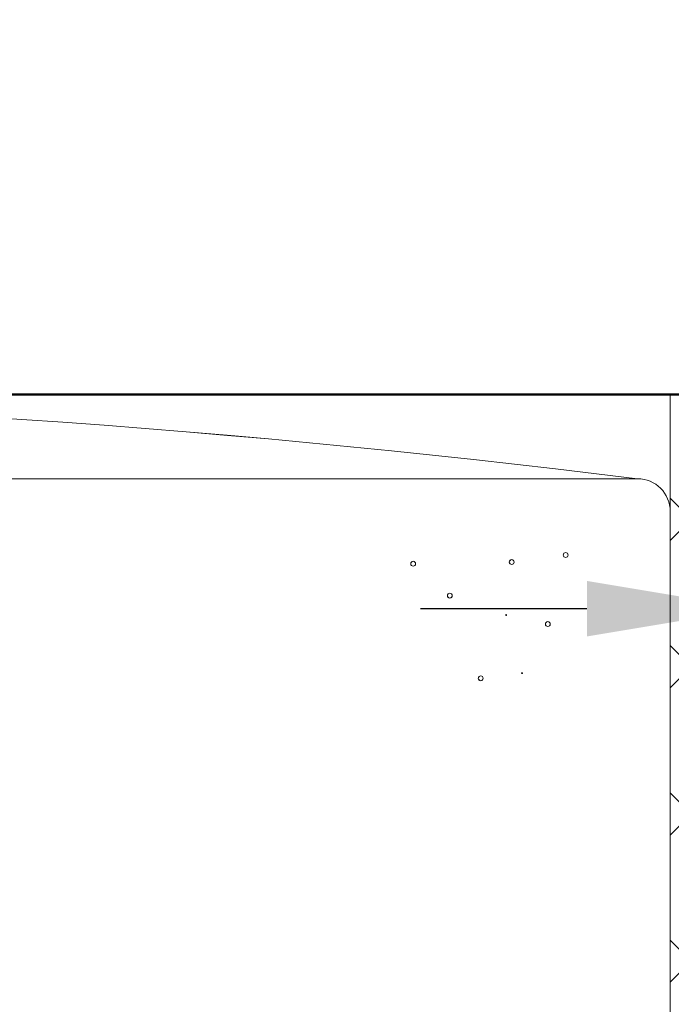
# Model space of a CAD drawing. Units: inches. Extents: x -466983 to 1020, y 324 to 318697.
# Tile 84 of 97: x 663 to 679, y 939 to 963. Entities that reach past the tile are written whole.
import ezdxf

# ---------------------------------------------------------------- set-up
doc = ezdxf.new("R2010")
doc.units = ezdxf.units.IN
doc.header["$MEASUREMENT"] = 0
for name, color, linetype, lineweight in [('A-ANNO-DIMS', 2, 'Continuous', 18), ('A-FLOR-PATT', 252, 'Continuous', 13), ('A-FURN', 8, 'Continuous', 18), ('A-WALL', 7, 'Continuous', 50)]:
    doc.layers.add(name, color=color, linetype=linetype, lineweight=lineweight)
doc.styles.get("Standard").update_dxf_attribs({"font": 'arial.ttf'})
doc.dimstyles.get("Standard").update_dxf_attribs({"dimtxt": 6, "dimasz": 4, "dimexe": 3, "dimexo": 3, "dimgap": 0.09, "dimtad": 0, "dimtih": 1, "dimtoh": 1, "dimdec": 1, "dimzin": 0, "dimdsep": 46, "dimlunit": 3, "dimtxsty": 'Standard', "dimcen": 0.09, "dimadec": 0, "dimazin": 0, "dimtfac": 1, "dimtdec": 1, "dimtofl": 0, "dimtmove": 0, "dimatfit": 3, "dimfxl": 1, "dimtolj": 1, "dimtzin": 0, "dimarcsym": 0})

# ---------------------------------------------------------------- blocks, each defined once
blk = doc.blocks.new('L Shaped Sofa')
at = {"ltscale": 2}
for p, q in [((2355.263, 760.482), (2355.263, 736.259)), ((2355.263, 728.35), (2355.263, 736.259)), ((2355.263, 723.229), (2355.263, 728.35)), ((2356.696, 726.917), (2377.232, 726.917)), ((2393.28, 726.917), (2377.232, 726.917)), ((2355.263, 723.229), (2377.232, 723.229)), ((2475.263, 723.229), (2377.232, 723.229))]:
    blk.add_line(p, q, dxfattribs=at)
for centre, radius, start, end in [((2363.564, 735.657), 0.106, 90, 270), ((2363.564, 735.657), 0.106, 270, 90), ((2361.755, 735.431), 0.0177, 90, 270), ((2361.755, 735.431), 0.0177, 270, 90), ((2360.624, 733.281), 0.106, 90, 270), ((2360.624, 733.281), 0.106, 270, 90), ((2362.453, 732.887), 0.0177, 90, 270), ((2362.453, 732.887), 0.0177, 270, 90), ((2364.92, 732.036), 0.106, 90, 270), ((2364.92, 732.036), 0.106, 270, 90), ((2362.207, 730.566), 0.106, 90, 270), ((2362.207, 730.566), 0.106, 270, 90), ((2366.526, 730.64), 0.106, 90, 270), ((2366.526, 730.64), 0.106, 270, 90), ((2359.842, 730.258), 0.106, 90, 270), ((2359.842, 730.258), 0.106, 270, 90), ((2356.696, 728.35), 1.433, 180, 270), ((2416.36, 1205.029), 481.82, 262.88673, 276.63201)]:
    blk.add_arc(centre, radius, start, end, dxfattribs=at)
blk = doc.blocks.new('*D58')
at = {"layer": 'A-ANNO-DIMS', "color": 0, "lineweight": -2, "transparency": 16777216}
for p, q in [((680.592, 950.938), (680.592, 945.795)), ((710.403, 950.938), (710.403, 945.795)), ((676.592, 948.795), (672.592, 948.795)), ((714.403, 948.795), (718.403, 948.795))]:
    blk.add_line(p, q, dxfattribs=at)
at = {"layer": 'A-ANNO-DIMS', "color": 0, "transparency": 16777216}
for points in [[(676.592, 949.462), (676.592, 948.129), (680.592, 948.795)], [(714.403, 949.462), (714.403, 948.129), (710.403, 948.795)]]:
    blk.add_solid(points, dxfattribs=at)
at = {"layer": 'Defpoints', "color": 0, "transparency": 16777216}
for p in [(680.592, 953.938), (710.403, 953.938), (710.403, 948.795)]:
    blk.add_point(p, dxfattribs=at)
at = {"layer": 'A-ANNO-DIMS', "color": 0, "transparency": 16777216, "insert": (695.497, 948.795), "char_height": 6, "attachment_point": 5}
blk.add_mtext('\\A1;30 TYP.', dxfattribs=at)

msp = doc.modelspace()

# ---------------------------------------------------------------- hatches: boundary and pattern name
at = {"layer": 'A-FLOR-PATT', "transparency": 33554572}
h = msp.add_hatch(dxfattribs=at)
h.set_pattern_fill('ANSI37', color=256, scale=30)
h.set_pattern_definition([(45, (-1212.4137, -290.035), (-2.6516504, 2.6516504), []), (135, (-1212.4137, -290.035), (-2.6516504, -2.6516504), [])])
h.paths.add_polyline_path([(901.806, 1075.938), (900.614, 1075.938), (900.614, 1065.386), (899.391, 1065.386), (898.091, 1065.386), (892.836, 1058.71, -0.258377), (892.188, 1058.351), (879.985, 1058.351, -0.20177), (879.438, 1058.581), (874.081, 1065.386), (872.781, 1065.386), (871.558, 1065.386), (871.558, 1075.938), (813.806, 1075.938), (813.806, 1044.792), (832.395, 1044.792, -0.394795), (848.66, 1028.536), (848.66, 1009.938), (901.806, 1009.938), (901.806, 1015.938), (901.306, 1015.938), (871.306, 1015.938), (871.306, 1017.25), (871.334, 1017.25, -0.401453), (901.306, 1045.938), (901.806, 1045.938)])
edge = h.paths.add_edge_path(flags=16)
edge.add_line((847.773, 1068.949), (847.773, 1073.709))
edge.add_arc((849.227, 1073.709), 1.454, 90, 180, ccw=False)
edge.add_line((849.227, 1075.163), (864.492, 1075.163))
edge.add_arc((864.492, 1073.709), 1.454, 0, 90, ccw=False)
edge.add_line((865.946, 1073.709), (865.946, 1069.004))
edge.add_arc((832.645, 1068.976), 33.301, -20.6123, 0.0472, ccw=False)
edge.add_ellipse((856.859, 1058.48), major_axis=(0, 10.213), ratio=0.685919, start_angle=100.0088, end_angle=259.9912, ccw=False)
edge.add_arc((881.074, 1068.976), 33.301, 180.0472, 200.6123, ccw=False)
h.paths.add_polyline_path([(853.146, 1066.482), (853.146, 1066.453), (853.146, 1066.453, 0.433107), (852.917, 1066.685), (852.917, 1066.453), (853.146, 1066.453), (853.146, 1066.482), (853.088, 1066.612, 0.697939), (852.7, 1066.453), (852.7, 1066.453), (852.7, 1066.482), (852.917, 1067.001), (852.917, 1066.685, -0.396254)], flags=0)
h.paths.add_polyline_path([(861.019, 1066.482), (861.019, 1066.453), (861.019, 1066.453, 0.416404), (860.802, 1066.685), (860.802, 1066.453), (861.019, 1066.453), (861.019, 1066.482), (860.967, 1066.605, 0.713344), (860.573, 1066.453), (860.573, 1066.453), (860.573, 1066.482), (860.802, 1067.001), (860.802, 1066.685, -0.379973)], flags=0)
edge = h.paths.add_edge_path(flags=0)
edge.add_spline(control_points=[(861.13, 1065.785), (861.466, 1065.248), (861.613, 1065.016), (861.983, 1064.374), (862.192, 1063.944), (862.561, 1063.039), (862.721, 1062.563), (862.987, 1061.578), (863.092, 1061.069), (863.245, 1060.031), (863.293, 1059.503), (863.329, 1058.441), (863.318, 1057.908), (863.237, 1056.852), (863.166, 1056.329), (862.97, 1055.308), (862.843, 1054.81), (862.537, 1053.852), (862.357, 1053.393), (861.951, 1052.525), (861.725, 1052.117), (861.233, 1051.362), (860.967, 1051.016), (860.405, 1050.395), (860.108, 1050.12), (859.494, 1049.646), (859.176, 1049.448), (858.528, 1049.13), (858.197, 1049.011), (857.531, 1048.852), (857.196, 1048.812), (856.525, 1048.812), (856.189, 1048.852), (855.524, 1049.01), (855.193, 1049.129), (854.545, 1049.447), (854.227, 1049.645), (853.612, 1050.118), (853.316, 1050.393), (852.753, 1051.014), (852.487, 1051.36), (851.995, 1052.114), (851.769, 1052.523), (851.363, 1053.39), (851.183, 1053.85), (850.877, 1054.807), (850.75, 1055.305), (850.553, 1056.326), (850.483, 1056.849), (850.401, 1057.905), (850.39, 1058.438), (850.426, 1059.5), (850.473, 1060.028), (850.626, 1061.066), (850.732, 1061.575), (850.997, 1062.561), (851.157, 1063.036), (851.525, 1063.942), (851.734, 1064.371), (852.106, 1065.016), (852.254, 1065.25), (852.608, 1065.733)], knot_values=[3.915332, 3.915332, 3.915332, 3.915332, 4.013468, 4.013468, 4.175532, 4.175532, 4.337596, 4.337596, 4.49966, 4.49966, 4.661724, 4.661724, 4.823788, 4.823788, 4.985852, 4.985852, 5.147916, 5.147916, 5.30998, 5.30998, 5.472044, 5.472044, 5.634109, 5.634109, 5.796173, 5.796173, 5.958237, 5.958237, 6.120301, 6.120301, 6.282365, 6.282365, 6.444429, 6.444429, 6.606493, 6.606493, 6.768557, 6.768557, 6.930621, 6.930621, 7.092685, 7.092685, 7.254749, 7.254749, 7.416813, 7.416813, 7.578878, 7.578878, 7.740942, 7.740942, 7.903006, 7.903006, 8.06507, 8.06507, 8.227134, 8.227134, 8.389198, 8.389198, 8.551262, 8.551262, 8.65037, 8.65037, 8.65037, 8.65037], degree=3, periodic=0)
edge.add_line((852.642, 1065.785), (861.13, 1065.785))
edge = h.paths.add_edge_path(flags=0)
edge.add_ellipse((856.85, 1057.743), major_axis=(0, 7.792), ratio=0.687861, start_angle=0, end_angle=360)
h.paths.add_polyline_path([(848.863, 1069.389), (848.863, 1073.96, -0.414214), (849.954, 1075.051), (863.765, 1075.051, -0.414214), (864.856, 1073.96), (864.856, 1069.389, -0.388936), (864.524, 1069.027, -0.043561), (849.195, 1069.027, -0.388936)], flags=0)
h.paths.add_polyline_path([(853.101, 1068.112, -1), (852.677, 1068.112, -1)], flags=0)
edge = h.paths.add_edge_path(flags=0)
edge.add_ellipse((856.859, 1057.338), major_axis=(0, 2.207), ratio=0.657164, start_angle=0, end_angle=360)
h.paths.add_polyline_path([(861.041, 1068.112, -1), (860.618, 1068.112, -1)], flags=0)
edge = h.paths.add_edge_path()
edge.add_line((573.954, 1057.341), (573.954, 1075.938))
edge.add_line((573.954, 1075.938), (558.731, 1075.938))
edge.add_line((558.731, 1075.938), (558.731, 1065.386))
edge.add_line((558.731, 1065.386), (557.507, 1065.386))
edge.add_line((557.507, 1065.386), (556.207, 1065.386))
edge.add_line((556.207, 1065.386), (550.952, 1058.71))
edge.add_arc((550.304, 1059.116), 0.765, 270, 327.9483, ccw=False)
edge.add_line((550.304, 1058.351), (538.101, 1058.351))
edge.add_arc((538.101, 1059.116), 0.765, 224.3704, 270, ccw=False)
edge.add_line((537.555, 1058.581), (532.198, 1065.386))
edge.add_line((532.198, 1065.386), (530.898, 1065.386))
edge.add_line((530.898, 1065.386), (529.674, 1065.386))
edge.add_line((529.674, 1065.386), (529.674, 1075.938))
edge.add_line((529.674, 1075.938), (520.806, 1075.938))
edge.add_line((520.806, 1075.938), (520.806, 1045.938))
edge.add_line((520.806, 1045.938), (521.306, 1045.938))
edge.add_arc((521.306, 1015.938), 30, 2.5075, 90, ccw=False)
edge.add_line((551.277, 1017.25), (551.306, 1017.25))
edge.add_line((551.306, 1017.25), (551.306, 1015.938))
edge.add_line((551.306, 1015.938), (520.806, 1015.938))
edge.add_line((520.806, 1015.938), (520.806, 1009.938))
edge.add_line((520.806, 1009.938), (559.191, 1010.402))
edge.add_arc((559.191, 1011.856), 1.454, 180, 270, ccw=False)
edge.add_line((557.737, 1011.856), (557.737, 1016.561))
edge.add_arc((591.039, 1016.589), 33.301, 159.3877, 180.0472, ccw=False)
edge.add_ellipse((566.824, 1027.085), major_axis=(0, 10.213), ratio=0.685919, start_angle=280.0088, end_angle=439.9912, ccw=False)
edge.add_arc((542.609, 1016.589), 33.301, 0.0472, 20.6123, ccw=False)
edge.add_line((575.91, 1016.616), (575.91, 1011.856))
edge.add_arc((574.456, 1011.856), 1.454, -90, 0, ccw=False)
edge.add_line((574.456, 1010.402), (608.806, 1009.938))
edge.add_line((608.806, 1009.938), (608.806, 1041.086))
edge.add_line((608.806, 1041.086), (590.218, 1041.086))
edge.add_arc((590.775, 1057.907), 16.831, 181.9277, 268.1032, ccw=False)
edge = h.paths.add_edge_path()
edge.add_ellipse((494.244, 583.62), major_axis=(0, 10.213), ratio=0.685919, start_angle=280.0088, end_angle=439.9912, ccw=False)
edge.add_arc((470.03, 573.124), 33.301, 0.0472, 20.6123, ccw=False)
edge.add_line((503.331, 573.152), (503.331, 568.392))
edge.add_arc((501.877, 568.392), 1.454, -90, 0, ccw=False)
edge.add_line((501.877, 566.938), (539.806, 566.938))
edge.add_line((539.806, 566.938), (539.806, 572.938))
edge.add_line((539.806, 572.938), (539.306, 572.938))
edge.add_line((539.306, 572.938), (509.306, 572.938))
edge.add_line((509.306, 572.938), (509.306, 574.25))
edge.add_line((509.306, 574.25), (509.334, 574.25))
edge.add_arc((539.306, 572.938), 30, 90, 177.4925, ccw=False)
edge.add_line((539.306, 602.938), (539.806, 602.938))
edge.add_line((539.806, 602.938), (539.806, 626.938))
edge.add_line((539.806, 626.938), (531.772, 626.938))
edge.add_line((531.772, 626.938), (531.772, 616.386))
edge.add_line((531.772, 616.386), (530.548, 616.386))
edge.add_line((530.548, 616.386), (529.249, 616.386))
edge.add_line((529.249, 616.386), (523.711, 609.351))
edge.add_line((523.711, 609.351), (510.777, 609.351))
edge.add_line((510.777, 609.351), (505.239, 616.386))
edge.add_line((505.239, 616.386), (503.939, 616.386))
edge.add_line((503.939, 616.386), (502.715, 616.386))
edge.add_line((502.715, 616.386), (502.715, 626.938))
edge.add_line((502.715, 626.938), (481.698, 626.938))
edge.add_line((481.698, 626.938), (481.698, 610.995))
edge.add_arc((467.27, 611.473), 14.436, 271.9277, 358.1032, ccw=False)
edge.add_line((467.756, 597.045), (451.806, 597.045))
edge.add_line((451.806, 597.045), (451.806, 584.404))
edge.add_line((451.806, 584.404), (451.806, 566.938))
edge.add_line((451.806, 566.938), (486.612, 566.938))
edge.add_arc((486.612, 568.392), 1.454, 180, 270, ccw=False)
edge.add_line((485.158, 568.392), (485.158, 573.097))
edge.add_arc((518.459, 573.124), 33.301, 159.3877, 180.0472, ccw=False)
h.paths.add_polyline_path([(836.261, 1020.733), (879.89, 1020.733), (879.89, 1039.39), (836.261, 1039.39)], flags=25)
h.paths.add_polyline_path([(549.985, 1036.749), (593.614, 1036.749), (593.614, 1055.407), (549.985, 1055.407)], flags=24)
h.paths.add_polyline_path([(475.123, 595.596), (518.752, 595.596), (518.752, 614.253), (475.123, 614.253)], flags=24)
h = msp.add_hatch(dxfattribs=at)
h.set_pattern_fill('ANSI37', color=256, scale=20)
h.set_pattern_definition([(45, (-1212.4137, -290.035), (-1.767767, 1.767767), []), (135, (-1212.4137, -290.035), (-1.767767, -1.767767), [])])
h.paths.add_polyline_path([(809.806, 870.938), (809.806, 888.152), (806.998, 888.152), (802.662, 888.152), (789.383, 888.152), (786.285, 888.152, -0.414214), (785.499, 888.937), (785.499, 900.196), (785.499, 908.47, -0.414214), (786.808, 909.779, -0.414214), (785.499, 911.088), (785.499, 929.101, -0.414214), (786.808, 930.411, -0.414214), (785.499, 931.72), (785.499, 931.904, -0.414214), (784.19, 930.595), (766.722, 930.595, -0.412359), (765.413, 931.896, -0.413741), (764.115, 930.578), (744.578, 930.422, -0.416556), (743.786, 931.207), (743.786, 933.515), (742.215, 933.515), (742.215, 952.024, -0.001344), (743.786, 952.2), (743.786, 953.938), (678.592, 953.938), (678.592, 951.131), (678.592, 946.794), (678.592, 933.515), (678.592, 930.417, -0.414214), (677.806, 929.631), (666.548, 929.631), (658.274, 929.631, -0.414214), (656.965, 930.94, -0.414214), (655.656, 929.631), (637.642, 929.631, -0.414214), (636.333, 930.94, -0.414214), (635.024, 929.631), (634.839, 929.631, -0.414214), (636.149, 928.322), (636.149, 910.854, -0.412359), (634.848, 909.545, -0.413741), (636.165, 908.247), (636.321, 888.71, -0.416556), (635.536, 887.918), (633.228, 887.918), (633.228, 886.347), (614.719, 886.347, -0.001344), (614.544, 887.918), (612.806, 887.918), (612.806, 834.938), (612.806, 752.938), (612.806, 748.938), (612.806, 697.938), (654.806, 697.938), (654.806, 701.938), (715.806, 701.938), (715.806, 737.435), (774.292, 737.435), (774.292, 795.938), (809.806, 795.938)])
h.paths.add_polyline_path([(679.276, 849.576, 0.102523), (682.148, 849.261, -0.080461), (694.543, 849.773, -0.283899), (694.482, 849.008, 0.136605), (694.407, 848.81, -0.030441), (694.543, 846.893), (694.543, 842.62), (694.543, 838.347, -0.028219), (694.425, 836.568), (694.425, 836.568, 0.196187), (694.446, 836.271, -0.302897), (694.543, 835.467, -0.080461), (682.148, 835.979, 0.102523), (679.276, 835.664, -0.58611), (678.646, 836.017), (678.646, 849.223, -0.58611)], flags=16)
h.paths.add_polyline_path([(679.517, 848.651, 0.699597), (679.476, 848.634, 1.20716), (679.194, 848.742, 0.010621)], flags=0)
h.paths.add_polyline_path([(679.492, 836.561, -0.013798), (679.918, 836.659, -0.071703), (682.853, 837.143, -0.165743), (682.166, 839.101), (682.166, 842.609), (682.166, 846.06, -0.240616), (683.473, 848.677, -0.068263), (693.929, 849.008), (693.788, 848.708), (693.788, 849.023, 0.067332), (683.473, 848.677, 0.240616), (682.166, 846.06), (682.166, 842.609), (682.166, 839.101, 0.23459), (683.461, 836.551, 0.068093), (693.788, 836.195), (693.788, 836.51), (693.93, 836.21, -0.077215), (682.242, 836.782, 0.086627), (679.528, 836.57, -0.628402), (679.503, 836.573), (679.503, 836.607, 0.910458)], flags=0)
h.paths.add_polyline_path([(679.476, 848.636), (679.207, 848.647), (679.207, 836.572, 0.913566), (679.365, 836.586), (679.476, 836.582)], flags=0)
h.paths.add_polyline_path([(679.276, 829.86, 0.102523), (682.148, 829.546, -0.080461), (694.543, 830.057, -0.283899), (694.482, 829.293, 0.136605), (694.407, 829.095, -0.030441), (694.543, 827.178), (694.543, 822.904), (694.543, 818.631, -0.028219), (694.425, 816.853), (694.425, 816.853, 0.196187), (694.446, 816.556, -0.302897), (694.543, 815.752, -0.080461), (682.148, 816.263, 0.102523), (679.276, 815.949, -0.58611), (678.646, 816.302), (678.646, 829.507, -0.58611)], flags=16)
h.paths.add_polyline_path([(679.517, 828.936, 0.699597), (679.476, 828.919, 1.20716), (679.194, 829.027, 0.010621)], flags=0)
h.paths.add_polyline_path([(679.492, 816.846, -0.013798), (679.918, 816.944, -0.071703), (682.853, 817.428, -0.165743), (682.166, 819.385), (682.166, 822.894), (682.166, 826.345, -0.240616), (683.473, 828.961, -0.068263), (693.929, 829.293), (693.788, 828.993), (693.788, 829.308, 0.067332), (683.473, 828.961, 0.240616), (682.166, 826.345), (682.166, 822.894), (682.166, 819.385, 0.23459), (683.461, 816.836, 0.068093), (693.788, 816.48), (693.788, 816.795), (693.93, 816.495, -0.077215), (682.242, 817.066, 0.086627), (679.528, 816.855, -0.628402), (679.503, 816.858), (679.503, 816.892, 0.910458)], flags=0)
h.paths.add_polyline_path([(679.476, 828.921), (679.207, 828.932), (679.207, 816.857, 0.913566), (679.365, 816.871), (679.476, 816.867)], flags=0)
h.paths.add_polyline_path([(679.276, 810.145, 0.102523), (682.148, 809.83, -0.080461), (694.543, 810.342, -0.3023), (694.447, 809.539, 0.10023), (694.406, 809.388, -0.03057), (694.543, 807.462), (694.543, 803.189), (694.543, 798.916, -0.03057), (694.406, 796.991, 0.10023), (694.447, 796.839, -0.3023), (694.543, 796.036, -0.080461), (682.148, 796.548, 0.102523), (679.276, 796.233, -0.58611), (678.646, 796.586), (678.646, 809.792, -0.58611)], flags=16)
h.paths.add_polyline_path([(679.517, 809.242, 0.699597), (679.476, 809.224, 1.20716), (679.194, 809.332, 0.010621)], flags=0)
h.paths.add_polyline_path([(679.492, 797.151, -0.013798), (679.918, 797.25, -0.071703), (682.853, 797.734, -0.165743), (682.166, 799.691), (682.166, 803.2), (682.166, 806.65, -0.239349), (683.461, 809.258, -0.072465), (694.447, 809.541, 0.197932), (694.425, 809.241), (693.788, 809.299), (693.788, 809.614, 0.068093), (683.461, 809.258, 0.239349), (682.166, 806.65), (682.166, 803.2), (682.166, 799.691, 0.235854), (683.473, 797.132, 0.067332), (693.788, 796.786), (693.788, 797.101), (694.425, 797.159, 0.197932), (694.447, 796.859, -0.080419), (682.156, 797.379, 0.083867), (679.528, 797.16, -0.628402), (679.503, 797.164), (679.503, 797.197, 0.910458)], flags=0)
h.paths.add_polyline_path([(679.207, 809.237), (679.207, 797.162, 0.913566), (679.365, 797.176), (679.476, 797.173), (679.476, 809.227)], flags=0)
h.paths.add_polyline_path([(695.364, 853.299), (728.223, 853.299), (728.223, 771.152), (695.364, 771.152)], flags=16)
h.paths.add_polyline_path([(696.021, 852.642), (727.566, 852.642), (727.566, 771.809), (696.021, 771.809)], flags=0)
h.paths.add_polyline_path([(679.276, 788.787, 0.102523), (682.148, 788.472, -0.080461), (694.543, 788.984, -0.3023), (694.447, 788.181, 0.10023), (694.406, 788.03, -0.03057), (694.543, 786.104), (694.543, 781.831), (694.543, 777.558, -0.03057), (694.406, 775.632, 0.10023), (694.447, 775.481, -0.3023), (694.543, 774.678, -0.080461), (682.148, 775.19, 0.102523), (679.276, 774.875, -0.58611), (678.646, 775.228), (678.646, 788.434, -0.58611)], flags=16)
h.paths.add_polyline_path([(679.517, 787.883, 0.699597), (679.476, 787.866, 1.20716), (679.194, 787.974, 0.010621)], flags=0)
h.paths.add_polyline_path([(679.492, 775.793, -0.013798), (679.918, 775.891, -0.071703), (682.853, 776.375, -0.165743), (682.166, 778.333), (682.166, 781.841), (682.166, 785.292, -0.239349), (683.461, 787.899, -0.072465), (694.447, 788.182, 0.197932), (694.425, 787.882), (693.788, 787.94), (693.788, 788.255, 0.068093), (683.461, 787.899, 0.239349), (682.166, 785.292), (682.166, 781.841), (682.166, 778.333, 0.235854), (683.473, 775.774, 0.067332), (693.788, 775.428), (693.788, 775.742), (694.425, 775.8, 0.197932), (694.447, 775.5, -0.080419), (682.156, 776.021, 0.083867), (679.528, 775.802, -0.628402), (679.503, 775.805), (679.503, 775.839, 0.910458)], flags=0)
h.paths.add_polyline_path([(679.207, 787.879), (679.207, 775.804, 0.913566), (679.365, 775.818), (679.476, 775.814), (679.476, 787.868)], flags=0)
h.paths.add_polyline_path([(704.641, 854.12, -0.080461), (705.153, 866.516, 0.102523), (704.838, 869.387, -0.58611), (705.191, 870.017), (718.397, 870.017, -0.58611), (718.75, 869.387, 0.102523), (718.435, 866.516, -0.080461), (718.946, 854.12, -0.3023), (718.144, 854.217, 0.10023), (717.992, 854.257, -0.03057), (716.067, 854.12), (711.794, 854.12), (707.521, 854.12, -0.03057), (705.595, 854.257, 0.10023), (705.444, 854.217, -0.3023)], flags=16)
h.paths.add_polyline_path([(717.846, 869.146, 0.699597), (717.829, 869.187, 1.20716), (717.937, 869.47, 0.010621)], flags=0)
h.paths.add_polyline_path([(705.463, 854.216, -0.080419), (705.984, 866.507, 0.083867), (705.765, 869.135, -0.628402), (705.768, 869.16), (705.802, 869.16, 0.910458), (705.756, 869.171, -0.013798), (705.854, 868.745, -0.071703), (706.338, 865.81, -0.165743), (708.295, 866.497), (711.804, 866.497), (715.255, 866.497, -0.239349), (717.862, 865.202, -0.072465), (718.145, 854.216, 0.197932), (717.845, 854.238), (717.903, 854.876), (718.218, 854.876, 0.068093), (717.862, 865.202, 0.239349), (715.255, 866.497), (711.804, 866.497), (708.295, 866.497, 0.235854), (705.737, 865.19, 0.067332), (705.391, 854.876), (705.705, 854.876), (705.763, 854.238, 0.197932)], flags=16)
h.paths.add_polyline_path([(705.766, 869.456, 0.913566), (705.781, 869.299), (705.777, 869.187), (717.831, 869.187), (717.842, 869.456)], flags=0)
h.paths.add_polyline_path([(729.045, 842.62), (729.045, 846.893, -0.03057), (729.182, 848.818, 0.10023), (729.141, 848.97, -0.3023), (729.045, 849.773, -0.080461), (741.44, 849.261, 0.102523), (744.311, 849.576, -0.58611), (744.942, 849.223), (744.942, 836.017, -0.58611), (744.311, 835.664, 0.102523), (741.44, 835.979, -0.080461), (729.045, 835.467, -0.3023), (729.141, 836.27, 0.10023), (729.182, 836.421, -0.03057), (729.045, 838.347)], flags=16)
h.paths.add_polyline_path([(744.111, 836.585, 1.20716), (744.394, 836.477, 0.010621), (744.07, 836.567, 0.699597)], flags=0)
h.paths.add_polyline_path([(729.141, 836.268, 0.197932), (729.162, 836.568), (729.8, 836.51), (729.8, 836.195, 0.068093), (740.126, 836.551, 0.239349), (741.421, 839.159), (741.421, 842.609), (741.421, 846.118, 0.235854), (740.114, 848.677, 0.067332), (729.8, 849.023), (729.8, 848.708), (729.162, 848.65, 0.197932), (729.141, 848.95, -0.080419), (741.432, 848.43, 0.083867), (744.059, 848.649, -0.628402), (744.085, 848.645), (744.085, 848.612, 0.910458), (744.095, 848.658, -0.013798), (743.67, 848.559, -0.071703), (740.734, 848.075, -0.165743), (741.421, 846.118), (741.421, 842.609), (741.421, 839.159, -0.239349), (740.126, 836.551, -0.072465)], flags=0)
h.paths.add_polyline_path([(729.045, 830.057, -0.080461), (741.44, 829.546, 0.102523), (744.311, 829.86, -0.58611), (744.942, 829.507), (744.942, 816.302, -0.58611), (744.311, 815.949, 0.102523), (741.44, 816.263, -0.080461), (729.045, 815.752, -0.3023), (729.141, 816.554, 0.10023), (729.182, 816.706, -0.03057), (729.045, 818.631), (729.045, 822.904), (729.045, 827.178, -0.03057), (729.182, 829.103, 0.10023), (729.141, 829.255, -0.3023)], flags=16)
h.paths.add_polyline_path([(744.111, 816.869, 1.20716), (744.394, 816.761, 0.010621), (744.07, 816.852, 0.699597)], flags=0)
h.paths.add_polyline_path([(729.141, 829.235, -0.080419), (741.432, 828.714, 0.083867), (744.059, 828.933, -0.628402), (744.085, 828.93), (744.085, 828.896, 0.910458), (744.095, 828.943, -0.013798), (743.67, 828.844, -0.071703), (740.734, 828.36, -0.165743), (741.421, 826.403), (741.421, 822.894), (741.421, 819.443, -0.239349), (740.126, 816.836, -0.072465), (729.141, 816.553, 0.197932), (729.162, 816.853), (729.8, 816.795), (729.8, 816.48, 0.068093), (740.126, 816.836, 0.239349), (741.421, 819.443), (741.421, 822.894), (741.421, 826.403, 0.235854), (740.114, 828.961, 0.067332), (729.8, 829.308), (729.8, 828.993), (729.162, 828.935, 0.197932)], flags=16)
h.paths.add_polyline_path([(729.045, 810.342, -0.080461), (741.44, 809.83, 0.102523), (744.311, 810.145, -0.58611), (744.942, 809.792), (744.942, 796.586, -0.58611), (744.311, 796.233, 0.102523), (741.44, 796.548, -0.080461), (729.045, 796.036, -0.283899), (729.105, 796.801, 0.136605), (729.181, 796.999, -0.030441), (729.045, 798.916), (729.045, 803.189), (729.045, 807.462, -0.028219), (729.163, 809.241), (729.162, 809.241, 0.196187), (729.142, 809.538, -0.302897)], flags=16)
h.paths.add_polyline_path([(744.111, 797.175, 1.20716), (744.394, 797.067, 0.010621), (744.07, 797.158, 0.699597)], flags=0)
h.paths.add_polyline_path([(741.345, 809.027, 0.086627), (744.059, 809.239, -0.628402), (744.085, 809.235), (744.085, 809.202, 0.910458), (744.095, 809.248, -0.013798), (743.67, 809.15, -0.071703), (740.734, 808.666, -0.165743), (741.421, 806.708), (741.421, 803.2), (741.421, 799.749, -0.240616), (740.114, 797.132, -0.068263), (729.658, 796.801), (729.8, 797.101), (729.8, 796.786, 0.067332), (740.114, 797.132, 0.240616), (741.421, 799.749), (741.421, 803.2), (741.421, 806.708, 0.23459), (740.126, 809.258, 0.068093), (729.8, 809.614), (729.8, 809.299), (729.658, 809.599, -0.077215)], flags=0)
h.paths.add_polyline_path([(704.641, 770.33, -0.283899), (705.405, 770.27, 0.136605), (705.603, 770.194, -0.030441), (707.521, 770.33), (711.794, 770.33), (716.067, 770.33, -0.028219), (717.845, 770.212), (717.845, 770.213, 0.196187), (718.143, 770.233, -0.302897), (718.946, 770.33, -0.080461), (718.435, 757.935, 0.102523), (718.75, 755.064, -0.58611), (718.397, 754.433), (705.191, 754.433, -0.58611), (704.838, 755.064, 0.102523), (705.153, 757.935, -0.080461)], flags=16)
h.paths.add_polyline_path([(705.762, 755.305, 0.699597), (705.779, 755.264, 1.20716), (705.671, 754.981, 0.010621)], flags=0)
h.paths.add_polyline_path([(705.405, 769.717), (705.705, 769.575), (705.391, 769.575, 0.067332), (705.737, 759.261, 0.240616), (708.353, 757.954), (711.804, 757.954), (715.313, 757.954, 0.23459), (717.862, 759.249, 0.068093), (718.218, 769.575), (717.903, 769.575), (718.203, 769.717, -0.077215), (717.632, 758.03, 0.086627), (717.843, 755.316, -0.628402), (717.84, 755.29), (717.806, 755.29, 0.910458), (717.853, 755.28, -0.013798), (717.754, 755.705, -0.071703), (717.27, 758.641, -0.165743), (715.313, 757.954), (711.804, 757.954), (708.353, 757.954, -0.240616), (705.737, 759.261, -0.068263)], flags=0)
h.paths.add_polyline_path([(729.045, 788.984, -0.080461), (741.44, 788.472, 0.102523), (744.311, 788.787, -0.58611), (744.942, 788.434), (744.942, 775.228, -0.58611), (744.311, 774.875, 0.102523), (741.44, 775.19, -0.080461), (729.045, 774.678, -0.283899), (729.105, 775.443, 0.136605), (729.181, 775.64, -0.030441), (729.045, 777.558), (729.045, 781.831), (729.045, 786.104, -0.028219), (729.163, 787.882), (729.162, 787.882, 0.196187), (729.142, 788.18, -0.302897)], flags=16)
h.paths.add_polyline_path([(744.111, 775.817, 1.20716), (744.394, 775.709, 0.010621), (744.07, 775.799, 0.699597)], flags=0)
h.paths.add_polyline_path([(741.345, 787.669, 0.086627), (744.059, 787.881, -0.628402), (744.085, 787.877), (744.085, 787.844, 0.910458), (744.095, 787.89, -0.013798), (743.67, 787.791, -0.071703), (740.734, 787.307, -0.165743), (741.421, 785.35), (741.421, 781.841), (741.421, 778.39, -0.240616), (740.114, 775.774, -0.068263), (729.658, 775.443), (729.8, 775.742), (729.8, 775.428, 0.067332), (740.114, 775.774, 0.240616), (741.421, 778.39), (741.421, 781.841), (741.421, 785.35, 0.23459), (740.126, 787.899, 0.068093), (729.8, 788.255), (729.8, 787.94), (729.658, 788.241, -0.077215)], flags=0)
h.paths.add_polyline_path([(744.111, 848.636), (744.111, 836.582), (744.381, 836.572), (744.381, 848.647, 0.913566), (744.223, 848.633)], flags=0)
h.paths.add_polyline_path([(744.223, 828.917), (744.111, 828.921), (744.111, 816.867), (744.381, 816.857), (744.381, 828.932, 0.913566)], flags=0)
h.paths.add_polyline_path([(717.831, 755.264), (705.777, 755.264), (705.766, 754.994), (717.842, 754.994, 0.913566), (717.827, 755.152)], flags=0)
h.paths.add_polyline_path([(744.223, 809.223), (744.111, 809.227), (744.111, 797.173), (744.381, 797.162), (744.381, 809.237, 0.913566)], flags=0)
h.paths.add_polyline_path([(744.111, 787.868), (744.111, 775.814), (744.381, 775.804), (744.381, 787.879, 0.913566), (744.223, 787.865)], flags=0)
h.paths.add_polyline_path([(678.877, 877.123), (737.613, 877.123), (737.613, 899.512), (678.877, 899.512)], flags=24)

# ---------------------------------------------------------------- linework, layer by layer
at = {"layer": 'A-FURN', "ltscale": 2}
for p, q in [((612.806, 953.938), (666.548, 953.938)), ((612.806, 953.938), (666.548, 953.938)), ((612.806, 953.938), (666.548, 953.938)), ((612.806, 953.938), (666.548, 953.938)), ((612.806, 953.938), (666.548, 953.938)), ((612.806, 953.938), (666.548, 953.938)), ((678.592, 953.938), (666.548, 953.938)), ((678.592, 953.938), (666.548, 953.938)), ((678.592, 953.938), (666.548, 953.938)), ((678.592, 953.938), (666.548, 953.938)), ((678.592, 953.938), (666.548, 953.938)), ((678.592, 953.938), (666.548, 953.938)), ((678.592, 953.938), (678.592, 951.131)), ((678.592, 953.938), (678.592, 951.131)), ((678.592, 953.938), (678.592, 951.131)), ((678.592, 953.938), (678.592, 951.131)), ((678.592, 953.938), (678.592, 951.131)), ((678.592, 953.938), (678.592, 951.131)), ((657.75, 951.916), (666.548, 951.916)), ((657.75, 951.916), (666.548, 951.916)), ((657.75, 951.916), (666.548, 951.916)), ((657.75, 951.916), (666.548, 951.916)), ((657.75, 951.916), (666.548, 951.916)), ((657.75, 951.916), (666.548, 951.916)), ((677.806, 951.916), (666.548, 951.916)), ((677.806, 951.916), (666.548, 951.916)), ((677.806, 951.916), (666.548, 951.916)), ((677.806, 951.916), (666.548, 951.916)), ((677.806, 951.916), (666.548, 951.916)), ((677.806, 951.916), (666.548, 951.916)), ((678.592, 951.131), (678.592, 946.794)), ((678.592, 951.131), (678.592, 946.794)), ((678.592, 951.131), (678.592, 946.794)), ((678.592, 951.131), (678.592, 946.794)), ((678.592, 951.131), (678.592, 946.794)), ((678.592, 951.131), (678.592, 946.794)), ((678.592, 933.515), (678.592, 946.794)), ((678.592, 933.515), (678.592, 946.794)), ((678.592, 933.515), (678.592, 946.794)), ((678.592, 933.515), (678.592, 946.794)), ((678.592, 933.515), (678.592, 946.794)), ((678.592, 933.515), (678.592, 946.794))]:
    msp.add_line(p, q, dxfattribs=at)
for centre, radius, start, end in [((645.097, 689.808), 264.141, 82.88673, 96.63201), ((645.097, 689.808), 264.141, 82.88673, 96.63201), ((645.097, 689.808), 264.141, 82.88673, 96.63201), ((645.097, 689.808), 264.141, 82.88673, 96.63201), ((645.097, 689.808), 264.141, 82.88673, 96.63201), ((645.097, 689.808), 264.141, 82.88673, 96.63201), ((677.806, 951.131), 0.785, 0, 90), ((677.806, 951.131), 0.785, 0, 90), ((677.806, 951.131), 0.785, 0, 90), ((677.806, 951.131), 0.785, 0, 90), ((677.806, 951.131), 0.785, 0, 90), ((677.806, 951.131), 0.785, 0, 90), ((676.081, 950.085), 0.0582, 90, 270), ((676.081, 950.085), 0.0582, 90, 270), ((676.081, 950.085), 0.0582, 90, 270), ((676.081, 950.085), 0.0582, 90, 270), ((676.081, 950.085), 0.0582, 90, 270), ((676.081, 950.085), 0.0582, 90, 270), ((676.081, 950.085), 0.0582, 270, 90), ((676.081, 950.085), 0.0582, 270, 90), ((676.081, 950.085), 0.0582, 270, 90), ((676.081, 950.085), 0.0582, 270, 90), ((676.081, 950.085), 0.0582, 270, 90), ((676.081, 950.085), 0.0582, 270, 90), ((672.417, 949.875), 0.0582, 90, 270), ((672.417, 949.875), 0.0582, 90, 270), ((672.417, 949.875), 0.0582, 90, 270), ((672.417, 949.875), 0.0582, 90, 270), ((672.417, 949.875), 0.0582, 90, 270), ((672.417, 949.875), 0.0582, 90, 270), ((672.417, 949.875), 0.0582, 270, 90), ((672.417, 949.875), 0.0582, 270, 90), ((672.417, 949.875), 0.0582, 270, 90), ((672.417, 949.875), 0.0582, 270, 90), ((672.417, 949.875), 0.0582, 270, 90), ((672.417, 949.875), 0.0582, 270, 90), ((674.785, 949.916), 0.0582, 90, 270), ((674.785, 949.916), 0.0582, 90, 270), ((674.785, 949.916), 0.0582, 90, 270), ((674.785, 949.916), 0.0582, 90, 270), ((674.785, 949.916), 0.0582, 90, 270), ((674.785, 949.916), 0.0582, 90, 270), ((674.785, 949.916), 0.0582, 270, 90), ((674.785, 949.916), 0.0582, 270, 90), ((674.785, 949.916), 0.0582, 270, 90), ((674.785, 949.916), 0.0582, 270, 90), ((674.785, 949.916), 0.0582, 270, 90), ((674.785, 949.916), 0.0582, 270, 90), ((673.297, 949.11), 0.0582, 90, 270), ((673.297, 949.11), 0.0582, 90, 270), ((673.297, 949.11), 0.0582, 90, 270), ((673.297, 949.11), 0.0582, 90, 270), ((673.297, 949.11), 0.0582, 90, 270), ((673.297, 949.11), 0.0582, 90, 270), ((673.297, 949.11), 0.0582, 270, 90), ((673.297, 949.11), 0.0582, 270, 90), ((673.297, 949.11), 0.0582, 270, 90), ((673.297, 949.11), 0.0582, 270, 90), ((673.297, 949.11), 0.0582, 270, 90), ((673.297, 949.11), 0.0582, 270, 90), ((674.65, 948.643), 0.0097, 90, 270), ((674.65, 948.643), 0.0097, 90, 270), ((674.65, 948.643), 0.0097, 90, 270), ((674.65, 948.643), 0.0097, 90, 270), ((674.65, 948.643), 0.0097, 90, 270), ((674.65, 948.643), 0.0097, 90, 270), ((674.65, 948.643), 0.0097, 270, 90), ((674.65, 948.643), 0.0097, 270, 90), ((674.65, 948.643), 0.0097, 270, 90), ((674.65, 948.643), 0.0097, 270, 90), ((674.65, 948.643), 0.0097, 270, 90), ((674.65, 948.643), 0.0097, 270, 90), ((675.652, 948.427), 0.0582, 90, 270), ((675.652, 948.427), 0.0582, 90, 270), ((675.652, 948.427), 0.0582, 90, 270), ((675.652, 948.427), 0.0582, 90, 270), ((675.652, 948.427), 0.0582, 90, 270), ((675.652, 948.427), 0.0582, 90, 270), ((675.652, 948.427), 0.0582, 270, 90), ((675.652, 948.427), 0.0582, 270, 90), ((675.652, 948.427), 0.0582, 270, 90), ((675.652, 948.427), 0.0582, 270, 90), ((675.652, 948.427), 0.0582, 270, 90), ((675.652, 948.427), 0.0582, 270, 90), ((674.041, 947.125), 0.0582, 90, 270), ((674.041, 947.125), 0.0582, 90, 270), ((674.041, 947.125), 0.0582, 90, 270), ((674.041, 947.125), 0.0582, 90, 270), ((674.041, 947.125), 0.0582, 90, 270), ((674.041, 947.125), 0.0582, 90, 270), ((674.041, 947.125), 0.0582, 270, 90), ((674.041, 947.125), 0.0582, 270, 90), ((674.041, 947.125), 0.0582, 270, 90), ((674.041, 947.125), 0.0582, 270, 90), ((674.041, 947.125), 0.0582, 270, 90), ((674.041, 947.125), 0.0582, 270, 90), ((675.033, 947.249), 0.0097, 90, 270), ((675.033, 947.249), 0.0097, 90, 270), ((675.033, 947.249), 0.0097, 90, 270), ((675.033, 947.249), 0.0097, 90, 270), ((675.033, 947.249), 0.0097, 90, 270), ((675.033, 947.249), 0.0097, 90, 270), ((675.033, 947.249), 0.0097, 270, 90), ((675.033, 947.249), 0.0097, 270, 90), ((675.033, 947.249), 0.0097, 270, 90), ((675.033, 947.249), 0.0097, 270, 90), ((675.033, 947.249), 0.0097, 270, 90), ((675.033, 947.249), 0.0097, 270, 90)]:
    msp.add_arc(centre, radius, start, end, dxfattribs=at)
at = {"layer": 'A-WALL'}
msp.add_line((612.806, 953.938), (680.592, 953.938), dxfattribs=at)

# ---------------------------------------------------------------- block references
at = {"layer": 'A-FURN', "xscale": 0.5482153745360612, "yscale": 0.5482153745360612, "zscale": 0.5482153745360612, "rotation": 180}
msp.add_blockref('L Shaped Sofa', (1969.783, 1350.423), dxfattribs=at)

# ---------------------------------------------------------------- dimensions: what is measured, and where the dimension line sits
at = {"layer": 'A-ANNO-DIMS'}
dim = msp.add_linear_dim(base=(710.403, 948.795), p1=(680.592, 953.938), p2=(710.403, 953.938), text='<> TYP.', dimstyle='Standard', override={"dimdec": 0, "dimlfac": 1, "dimrnd": 0, "dimzin": 0, "dimdsep": 46, "dimlunit": 2}, dxfattribs=at)
dim.commit()
dim.dimension.update_dxf_attribs({"geometry": '*D58', "text_midpoint": (695.497, 948.795)})

doc.saveas('drawing.dxf')
